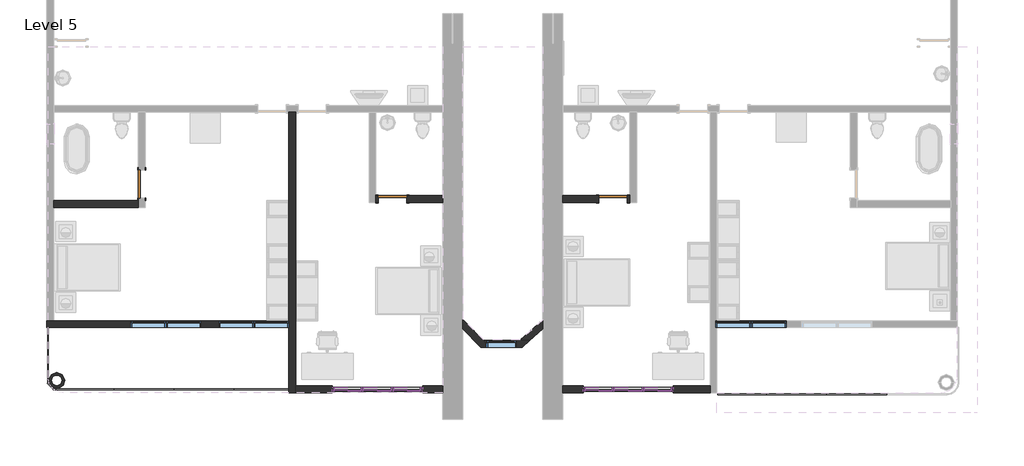
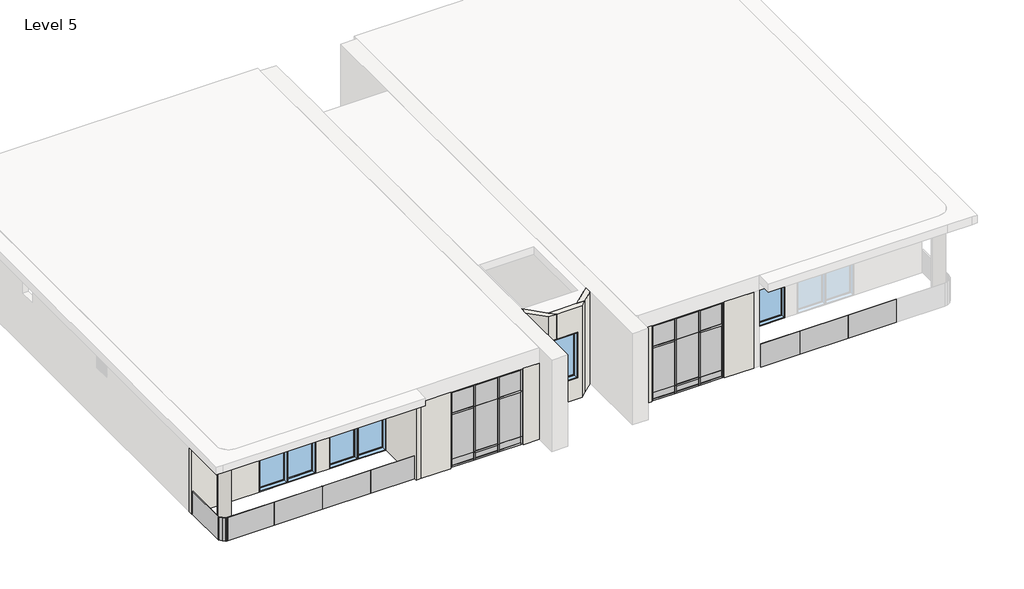
# One storey, part 1 of 3: 42 members, 30 plates, 14 walls, 7 windows, 3 doors.
"""IFC4 building model written with IfcOpenShell, lengths in millimetres."""

from ifc_helpers import new_model, si_unit, point, frame, frame_2d, origin, place, context, project, spatial, polyline, circle_curve, trimmed, segment, composite_curve, outline, extrude, faceted_brep, transform, mapped, element, save
from components import door_2703ae13, door_10fd3a06, member_c17f1be2, member_ad567e07, member_d2e7e466, member_7db1855a, member_75d1e245, member_d60e8053, member_3c3dc66a, member_2fae0574, member_410c6227, member_73c23c35, system_panel_glazed_38d54ecf, system_panel_glazed_fbb6c980, system_panel_glazed_4137532c, system_panel_glazed_6230de04, system_panel_glazed_a79f7f85, system_panel_glazed_9a5ea490, system_panel_glazed_95be5de7, system_panel_glazed_1e00a1c5, system_panel_glazed_ffe51582, system_panel_glazed_8f95e3f6, system_panel_glazed_836907cd, system_panel_glazed_688a65a2, system_panel_glazed_c1a1c740, system_panel_glazed_22bcd51f, window_9a779fa2, window_1a213a25

model = new_model("IFC4")

# Units and contexts
model_context = context("Model", 3, world=origin())
ifc_project = project(units=[si_unit("LENGTHUNIT", "METRE", prefix="MILLI")], contexts=[model_context])

# Site, building, storey
site = spatial("IfcSite", under=ifc_project)
building = spatial("IfcBuilding", under=site)
storey = spatial("IfcBuildingStorey", under=building, Name="Level 5", Elevation=14630.4)

# Doors
placement = place(None, origin())
door_shape = door_2703ae13(model_context)
element("IfcDoor", 1, ObjectType="Door-Single-Panel.0001 : 34\" x 80\"", at=placement, inside=storey, context=model_context, shape_type="MappedRepresentation", body=[
    mapped(door_shape, transform((-15765.9987704, -441.9241442, 14630.4), x_axis=(0.0, -1.0, 0.0), y_axis=(1.0, 0.0, 0.0), z_axis=(0.0, 0.0, 1.0))),
])
element("IfcDoor", 2, ObjectType="Door-Single-Panel.0001 : 34\" x 80\"", at=placement, inside=storey, context=model_context, shape_type="MappedRepresentation", body=[
    mapped(door_shape, transform((-8145.9987704, -899.1241442, 14630.4), x_axis=(-1.0, 0.0, 0.0), y_axis=(0.0, -1.0, 0.0), z_axis=(0.0, 0.0, 1.0))),
])
door_2_shape = door_10fd3a06(model_context)
element("IfcDoor", 3, ObjectType="Door-Single-Panel.0001 : 34\" x 80\"", at=placement, inside=storey, context=model_context, shape_type="MappedRepresentation", body=[
    mapped(door_2_shape, transform((-1440.3987704, -899.1241442, 14630.4), x_axis=(1.0, 0.0, 0.0), y_axis=(0.0, 1.0, 0.0), z_axis=(0.0, 0.0, 1.0))),
])

# Members
member_shape = member_c17f1be2(model_context)
element("IfcMember", 4, ObjectType="Rectangular Mullion : 2.5\" x 5\" rectangular", at=placement, inside=storey, context=model_context, shape_type="MappedRepresentation", body=[
    mapped(member_shape, transform((-9911.2987704, -6690.3241442, 17678.4), x_axis=(0.0, 0.0, 1.0), y_axis=(0.0, 1.0, 0.0), z_axis=(-1.0, 0.0, 0.0))),
])
element("IfcMember", 5, ObjectType="Rectangular Mullion : 2.5\" x 5\" rectangular", at=placement, inside=storey, context=model_context, shape_type="MappedRepresentation", body=[
    mapped(member_shape, transform((-8114.2487704, -6690.3241442, 17678.4), x_axis=(0.0, 0.0, 1.0), y_axis=(0.0, 1.0, 0.0), z_axis=(-1.0, 0.0, 0.0))),
])
element("IfcMember", 6, ObjectType="Rectangular Mullion : 2.5\" x 5\" rectangular", at=placement, inside=storey, context=model_context, shape_type="MappedRepresentation", body=[
    mapped(member_shape, transform((-2291.2987704, -6690.3241442, 17678.4), x_axis=(0.0, 0.0, 1.0), y_axis=(0.0, 1.0, 0.0), z_axis=(-1.0, 0.0, 0.0))),
])
element("IfcMember", 7, ObjectType="Rectangular Mullion : 2.5\" x 5\" rectangular", at=placement, inside=storey, context=model_context, shape_type="MappedRepresentation", body=[
    mapped(member_shape, transform((-494.2487704, -6690.3241442, 17678.4), x_axis=(0.0, 0.0, 1.0), y_axis=(0.0, 1.0, 0.0), z_axis=(-1.0, 0.0, 0.0))),
])
element("IfcMember", 8, ObjectType="Rectangular Mullion : 2.5\" x 5\" rectangular", at=placement, inside=storey, context=model_context, shape_type="MappedRepresentation", body=[
    mapped(member_shape, transform((-7295.0987704, -6690.3241442, 14630.4), x_axis=(0.0, 0.0, -1.0), y_axis=(0.0, 1.0, 0.0), z_axis=(1.0, 0.0, 0.0))),
])
element("IfcMember", 9, ObjectType="Rectangular Mullion : 2.5\" x 5\" rectangular", at=placement, inside=storey, context=model_context, shape_type="MappedRepresentation", body=[
    mapped(member_shape, transform((-9092.1487704, -6690.3241442, 14630.4), x_axis=(0.0, 0.0, -1.0), y_axis=(0.0, 1.0, 0.0), z_axis=(1.0, 0.0, 0.0))),
])
element("IfcMember", 10, ObjectType="Rectangular Mullion : 2.5\" x 5\" rectangular", at=placement, inside=storey, context=model_context, shape_type="MappedRepresentation", body=[
    mapped(member_shape, transform((324.9012296, -6690.3241442, 14630.4), x_axis=(0.0, 0.0, -1.0), y_axis=(0.0, 1.0, 0.0), z_axis=(1.0, 0.0, 0.0))),
])
element("IfcMember", 11, ObjectType="Rectangular Mullion : 2.5\" x 5\" rectangular", at=placement, inside=storey, context=model_context, shape_type="MappedRepresentation", body=[
    mapped(member_shape, transform((-1472.1487704, -6690.3241442, 14630.4), x_axis=(0.0, 0.0, -1.0), y_axis=(0.0, 1.0, 0.0), z_axis=(1.0, 0.0, 0.0))),
])
member_2_shape = member_ad567e07(model_context)
element("IfcMember", 12, ObjectType="Rectangular Mullion : 2.5\" x 5\" rectangular", at=placement, inside=storey, context=model_context, shape_type="MappedRepresentation", body=[
    mapped(member_2_shape, transform((-8114.2487704, -6690.3241442, 16764.0), x_axis=(0.0, 0.0, 1.0), y_axis=(0.0, 1.0, 0.0), z_axis=(-1.0, 0.0, 0.0))),
])
element("IfcMember", 13, ObjectType="Rectangular Mullion : 2.5\" x 5\" rectangular", at=placement, inside=storey, context=model_context, shape_type="MappedRepresentation", body=[
    mapped(member_2_shape, transform((-9911.2987704, -6690.3241442, 16764.0), x_axis=(0.0, 0.0, 1.0), y_axis=(0.0, 1.0, 0.0), z_axis=(-1.0, 0.0, 0.0))),
])
element("IfcMember", 14, ObjectType="Rectangular Mullion : 2.5\" x 5\" rectangular", at=placement, inside=storey, context=model_context, shape_type="MappedRepresentation", body=[
    mapped(member_2_shape, transform((-494.2487704, -6690.3241442, 16764.0), x_axis=(0.0, 0.0, 1.0), y_axis=(0.0, 1.0, 0.0), z_axis=(-1.0, 0.0, 0.0))),
])
element("IfcMember", 15, ObjectType="Rectangular Mullion : 2.5\" x 5\" rectangular", at=placement, inside=storey, context=model_context, shape_type="MappedRepresentation", body=[
    mapped(member_2_shape, transform((-2291.2987704, -6690.3241442, 16764.0), x_axis=(0.0, 0.0, 1.0), y_axis=(0.0, 1.0, 0.0), z_axis=(-1.0, 0.0, 0.0))),
])
member_3_shape = member_d2e7e466(model_context)
element("IfcMember", 16, ObjectType="Rectangular Mullion : 2.5\" x 5\" rectangular", at=placement, inside=storey, context=model_context, shape_type="MappedRepresentation", body=[
    mapped(member_3_shape, transform((-8177.7487704, -6690.3241442, 14630.4), x_axis=(0.0, 0.0, -1.0), y_axis=(0.0, 1.0, 0.0), z_axis=(1.0, 0.0, 0.0))),
])
element("IfcMember", 17, ObjectType="Rectangular Mullion : 2.5\" x 5\" rectangular", at=placement, inside=storey, context=model_context, shape_type="MappedRepresentation", body=[
    mapped(member_3_shape, transform((-557.7487704, -6690.3241442, 14630.4), x_axis=(0.0, 0.0, -1.0), y_axis=(0.0, 1.0, 0.0), z_axis=(1.0, 0.0, 0.0))),
])
member_4_shape = member_7db1855a(model_context)
element("IfcMember", 18, ObjectType="Rectangular Mullion : 2.5\" x 5\" rectangular", at=placement, inside=storey, context=model_context, shape_type="MappedRepresentation", body=[
    mapped(member_4_shape, transform((-9028.6487704, -6690.3241442, 14935.2), x_axis=(0.0, 0.0, 1.0), y_axis=(0.0, 1.0, 0.0), z_axis=(-1.0, 0.0, 0.0))),
])
element("IfcMember", 19, ObjectType="Rectangular Mullion : 2.5\" x 5\" rectangular", at=placement, inside=storey, context=model_context, shape_type="MappedRepresentation", body=[
    mapped(member_4_shape, transform((-1408.6487704, -6690.3241442, 14935.2), x_axis=(0.0, 0.0, 1.0), y_axis=(0.0, 1.0, 0.0), z_axis=(-1.0, 0.0, 0.0))),
])
element("IfcMember", 20, ObjectType="Rectangular Mullion : 2.5\" x 5\" rectangular", at=placement, inside=storey, context=model_context, shape_type="MappedRepresentation", body=[
    mapped(member_3_shape, transform((-9028.6487704, -6690.3241442, 17678.4), x_axis=(0.0, 0.0, 1.0), y_axis=(0.0, 1.0, 0.0), z_axis=(-1.0, 0.0, 0.0))),
])
element("IfcMember", 21, ObjectType="Rectangular Mullion : 2.5\" x 5\" rectangular", at=placement, inside=storey, context=model_context, shape_type="MappedRepresentation", body=[
    mapped(member_3_shape, transform((-1408.6487704, -6690.3241442, 17678.4), x_axis=(0.0, 0.0, 1.0), y_axis=(0.0, 1.0, 0.0), z_axis=(-1.0, 0.0, 0.0))),
])
member_5_shape = member_75d1e245(model_context)
element("IfcMember", 22, ObjectType="Rectangular Mullion : 2.5\" x 5\" rectangular", at=placement, inside=storey, context=model_context, shape_type="MappedRepresentation", body=[
    mapped(member_5_shape, transform((-8145.9987704, -6690.3241442, 14630.4), x_axis=(-1.0, 0.0, 0.0), y_axis=(0.0, 1.0, 0.0), z_axis=(0.0, 0.0, -1.0))),
])
element("IfcMember", 23, ObjectType="Rectangular Mullion : 2.5\" x 5\" rectangular", at=placement, inside=storey, context=model_context, shape_type="MappedRepresentation", body=[
    mapped(member_5_shape, transform((-9060.3987704, -6690.3241442, 14630.4), x_axis=(-1.0, 0.0, 0.0), y_axis=(0.0, 1.0, 0.0), z_axis=(0.0, 0.0, -1.0))),
])
element("IfcMember", 24, ObjectType="Rectangular Mullion : 2.5\" x 5\" rectangular", at=placement, inside=storey, context=model_context, shape_type="MappedRepresentation", body=[
    mapped(member_5_shape, transform((-525.9987704, -6690.3241442, 14630.4), x_axis=(-1.0, 0.0, 0.0), y_axis=(0.0, 1.0, 0.0), z_axis=(0.0, 0.0, -1.0))),
])
element("IfcMember", 25, ObjectType="Rectangular Mullion : 2.5\" x 5\" rectangular", at=placement, inside=storey, context=model_context, shape_type="MappedRepresentation", body=[
    mapped(member_5_shape, transform((-1440.3987704, -6690.3241442, 14630.4), x_axis=(-1.0, 0.0, 0.0), y_axis=(0.0, 1.0, 0.0), z_axis=(0.0, 0.0, -1.0))),
])
member_6_shape = member_d60e8053(model_context)
element("IfcMember", 26, ObjectType="Rectangular Mullion : 2.5\" x 5\" rectangular", at=placement, inside=storey, context=model_context, shape_type="MappedRepresentation", body=[
    mapped(member_6_shape, transform((-8145.9987704, -6690.3241442, 14935.2), x_axis=(-1.0, 0.0, 0.0), y_axis=(0.0, 1.0, 0.0), z_axis=(0.0, 0.0, -1.0))),
])
element("IfcMember", 27, ObjectType="Rectangular Mullion : 2.5\" x 5\" rectangular", at=placement, inside=storey, context=model_context, shape_type="MappedRepresentation", body=[
    mapped(member_6_shape, transform((-9060.3987704, -6690.3241442, 14935.2), x_axis=(-1.0, 0.0, 0.0), y_axis=(0.0, 1.0, 0.0), z_axis=(0.0, 0.0, -1.0))),
])
element("IfcMember", 28, ObjectType="Rectangular Mullion : 2.5\" x 5\" rectangular", at=placement, inside=storey, context=model_context, shape_type="MappedRepresentation", body=[
    mapped(member_6_shape, transform((-525.9987704, -6690.3241442, 14935.2), x_axis=(-1.0, 0.0, 0.0), y_axis=(0.0, 1.0, 0.0), z_axis=(0.0, 0.0, -1.0))),
])
element("IfcMember", 29, ObjectType="Rectangular Mullion : 2.5\" x 5\" rectangular", at=placement, inside=storey, context=model_context, shape_type="MappedRepresentation", body=[
    mapped(member_6_shape, transform((-1440.3987704, -6690.3241442, 14935.2), x_axis=(-1.0, 0.0, 0.0), y_axis=(0.0, 1.0, 0.0), z_axis=(0.0, 0.0, -1.0))),
])
member_7_shape = member_3c3dc66a(model_context)
element("IfcMember", 30, ObjectType="Rectangular Mullion : 2.5\" x 5\" rectangular", at=placement, inside=storey, context=model_context, shape_type="MappedRepresentation", body=[
    mapped(member_7_shape, transform((-9974.7987704, -6690.3241442, 14630.4), x_axis=(-1.0, 0.0, 0.0), y_axis=(0.0, 1.0, 0.0), z_axis=(0.0, 0.0, -1.0))),
])
element("IfcMember", 31, ObjectType="Rectangular Mullion : 2.5\" x 5\" rectangular", at=placement, inside=storey, context=model_context, shape_type="MappedRepresentation", body=[
    mapped(member_7_shape, transform((-2354.7987704, -6690.3241442, 14630.4), x_axis=(-1.0, 0.0, 0.0), y_axis=(0.0, 1.0, 0.0), z_axis=(0.0, 0.0, -1.0))),
])
member_8_shape = member_2fae0574(model_context)
element("IfcMember", 32, ObjectType="Rectangular Mullion : 2.5\" x 5\" rectangular", at=placement, inside=storey, context=model_context, shape_type="MappedRepresentation", body=[
    mapped(member_8_shape, transform((-9974.7987704, -6690.3241442, 14935.2), x_axis=(-1.0, 0.0, 0.0), y_axis=(0.0, 1.0, 0.0), z_axis=(0.0, 0.0, -1.0))),
])
element("IfcMember", 33, ObjectType="Rectangular Mullion : 2.5\" x 5\" rectangular", at=placement, inside=storey, context=model_context, shape_type="MappedRepresentation", body=[
    mapped(member_8_shape, transform((-2354.7987704, -6690.3241442, 14935.2), x_axis=(-1.0, 0.0, 0.0), y_axis=(0.0, 1.0, 0.0), z_axis=(0.0, 0.0, -1.0))),
])
element("IfcMember", 34, ObjectType="Rectangular Mullion : 2.5\" x 5\" rectangular", at=placement, inside=storey, context=model_context, shape_type="MappedRepresentation", body=[
    mapped(member_8_shape, transform((-7231.5987704, -6690.3241442, 16764.0), x_axis=(1.0, 0.0, 0.0), y_axis=(0.0, 1.0, 0.0), z_axis=(0.0, 0.0, 1.0))),
])
element("IfcMember", 35, ObjectType="Rectangular Mullion : 2.5\" x 5\" rectangular", at=placement, inside=storey, context=model_context, shape_type="MappedRepresentation", body=[
    mapped(member_8_shape, transform((388.4012296, -6690.3241442, 16764.0), x_axis=(1.0, 0.0, 0.0), y_axis=(0.0, 1.0, 0.0), z_axis=(0.0, 0.0, 1.0))),
])
element("IfcMember", 36, ObjectType="Rectangular Mullion : 2.5\" x 5\" rectangular", at=placement, inside=storey, context=model_context, shape_type="MappedRepresentation", body=[
    mapped(member_7_shape, transform((-7231.5987704, -6690.3241442, 14935.2), x_axis=(1.0, 0.0, 0.0), y_axis=(0.0, 1.0, 0.0), z_axis=(0.0, 0.0, 1.0))),
])
element("IfcMember", 37, ObjectType="Rectangular Mullion : 2.5\" x 5\" rectangular", at=placement, inside=storey, context=model_context, shape_type="MappedRepresentation", body=[
    mapped(member_7_shape, transform((388.4012296, -6690.3241442, 14935.2), x_axis=(1.0, 0.0, 0.0), y_axis=(0.0, 1.0, 0.0), z_axis=(0.0, 0.0, 1.0))),
])
member_9_shape = member_410c6227(model_context)
element("IfcMember", 38, ObjectType="Rectangular Mullion : 2.5\" x 5\" rectangular", at=placement, inside=storey, context=model_context, shape_type="MappedRepresentation", body=[
    mapped(member_9_shape, transform((-8145.9987704, -6690.3241442, 16764.0), x_axis=(-1.0, 0.0, 0.0), y_axis=(0.0, 1.0, 0.0), z_axis=(0.0, 0.0, -1.0))),
])
element("IfcMember", 39, ObjectType="Rectangular Mullion : 2.5\" x 5\" rectangular", at=placement, inside=storey, context=model_context, shape_type="MappedRepresentation", body=[
    mapped(member_9_shape, transform((-9060.3987704, -6690.3241442, 16764.0), x_axis=(-1.0, 0.0, 0.0), y_axis=(0.0, 1.0, 0.0), z_axis=(0.0, 0.0, -1.0))),
])
element("IfcMember", 40, ObjectType="Rectangular Mullion : 2.5\" x 5\" rectangular", at=placement, inside=storey, context=model_context, shape_type="MappedRepresentation", body=[
    mapped(member_9_shape, transform((-525.9987704, -6690.3241442, 16764.0), x_axis=(-1.0, 0.0, 0.0), y_axis=(0.0, 1.0, 0.0), z_axis=(0.0, 0.0, -1.0))),
])
element("IfcMember", 41, ObjectType="Rectangular Mullion : 2.5\" x 5\" rectangular", at=placement, inside=storey, context=model_context, shape_type="MappedRepresentation", body=[
    mapped(member_9_shape, transform((-1440.3987704, -6690.3241442, 16764.0), x_axis=(-1.0, 0.0, 0.0), y_axis=(0.0, 1.0, 0.0), z_axis=(0.0, 0.0, -1.0))),
])
member_10_shape = member_73c23c35(model_context)
element("IfcMember", 42, ObjectType="Rectangular Mullion : 2.5\" x 5\" rectangular", at=placement, inside=storey, context=model_context, shape_type="MappedRepresentation", body=[
    mapped(member_10_shape, transform((-7231.5987704, -6690.3241442, 17678.4), x_axis=(1.0, 0.0, 0.0), y_axis=(0.0, 1.0, 0.0), z_axis=(0.0, 0.0, 1.0))),
])
element("IfcMember", 43, ObjectType="Rectangular Mullion : 2.5\" x 5\" rectangular", at=placement, inside=storey, context=model_context, shape_type="MappedRepresentation", body=[
    mapped(member_10_shape, transform((388.4012296, -6690.3241442, 17678.4), x_axis=(1.0, 0.0, 0.0), y_axis=(0.0, 1.0, 0.0), z_axis=(0.0, 0.0, 1.0))),
])
element("IfcMember", 44, ObjectType="Rectangular Mullion : 2.5\" x 5\" rectangular", at=placement, inside=storey, context=model_context, shape_type="MappedRepresentation", body=[
    mapped(member_10_shape, transform((-9974.7987704, -6690.3241442, 16764.0), x_axis=(-1.0, 0.0, 0.0), y_axis=(0.0, 1.0, 0.0), z_axis=(0.0, 0.0, -1.0))),
])
element("IfcMember", 45, ObjectType="Rectangular Mullion : 2.5\" x 5\" rectangular", at=placement, inside=storey, context=model_context, shape_type="MappedRepresentation", body=[
    mapped(member_10_shape, transform((-2354.7987704, -6690.3241442, 16764.0), x_axis=(-1.0, 0.0, 0.0), y_axis=(0.0, 1.0, 0.0), z_axis=(0.0, 0.0, -1.0))),
])

# Plates
system_panel_glazed_shape = system_panel_glazed_38d54ecf(model_context)
element("IfcPlate", 46, ObjectType="System Panel : Glazed", at=placement, inside=storey, context=model_context, shape_type="MappedRepresentation", body=[
    mapped(system_panel_glazed_shape, transform((-8603.1987704, -6690.3241442, 14966.95), x_axis=(-1.0, 0.0, 0.0), y_axis=(0.0, -1.0, 0.0), z_axis=(0.0, 0.0, 1.0))),
])
element("IfcPlate", 47, ObjectType="System Panel : Glazed", at=placement, inside=storey, context=model_context, shape_type="MappedRepresentation", body=[
    mapped(system_panel_glazed_shape, transform((-983.1987704, -6690.3241442, 14966.95), x_axis=(-1.0, 0.0, 0.0), y_axis=(0.0, -1.0, 0.0), z_axis=(0.0, 0.0, 1.0))),
])
system_panel_glazed_2_shape = system_panel_glazed_fbb6c980(model_context)
element("IfcPlate", 48, ObjectType="System Panel : Glazed", at=placement, inside=storey, context=model_context, shape_type="MappedRepresentation", body=[
    mapped(system_panel_glazed_2_shape, transform((-8603.1987704, -6690.3241442, 14693.9), x_axis=(-1.0, 0.0, 0.0), y_axis=(0.0, -1.0, 0.0), z_axis=(0.0, 0.0, 1.0))),
])
element("IfcPlate", 49, ObjectType="System Panel : Glazed", at=placement, inside=storey, context=model_context, shape_type="MappedRepresentation", body=[
    mapped(system_panel_glazed_2_shape, transform((-983.1987704, -6690.3241442, 14693.9), x_axis=(-1.0, 0.0, 0.0), y_axis=(0.0, -1.0, 0.0), z_axis=(0.0, 0.0, 1.0))),
])
system_panel_glazed_3_shape = system_panel_glazed_4137532c(model_context)
element("IfcPlate", 50, ObjectType="System Panel : Glazed", at=placement, inside=storey, context=model_context, shape_type="MappedRepresentation", body=[
    mapped(system_panel_glazed_3_shape, transform((-7704.6737704, -6690.3241442, 14693.9), x_axis=(-1.0, 0.0, 0.0), y_axis=(0.0, -1.0, 0.0), z_axis=(0.0, 0.0, 1.0))),
])
element("IfcPlate", 51, ObjectType="System Panel : Glazed", at=placement, inside=storey, context=model_context, shape_type="MappedRepresentation", body=[
    mapped(system_panel_glazed_3_shape, transform((-9501.7237704, -6690.3241442, 14693.9), x_axis=(-1.0, 0.0, 0.0), y_axis=(0.0, -1.0, 0.0), z_axis=(0.0, 0.0, 1.0))),
])
element("IfcPlate", 52, ObjectType="System Panel : Glazed", at=placement, inside=storey, context=model_context, shape_type="MappedRepresentation", body=[
    mapped(system_panel_glazed_3_shape, transform((-84.6737704, -6690.3241442, 14693.9), x_axis=(-1.0, 0.0, 0.0), y_axis=(0.0, -1.0, 0.0), z_axis=(0.0, 0.0, 1.0))),
])
element("IfcPlate", 53, ObjectType="System Panel : Glazed", at=placement, inside=storey, context=model_context, shape_type="MappedRepresentation", body=[
    mapped(system_panel_glazed_3_shape, transform((-1881.7237704, -6690.3241442, 14693.9), x_axis=(-1.0, 0.0, 0.0), y_axis=(0.0, -1.0, 0.0), z_axis=(0.0, 0.0, 1.0))),
])
system_panel_glazed_4_shape = system_panel_glazed_6230de04(model_context)
element("IfcPlate", 54, ObjectType="System Panel : Glazed", at=placement, inside=storey, context=model_context, shape_type="MappedRepresentation", body=[
    mapped(system_panel_glazed_4_shape, transform((-7704.6737704, -6690.3241442, 14935.2), x_axis=(-1.0, 0.0, 0.0), y_axis=(0.0, -1.0, 0.0), z_axis=(0.0, 0.0, 1.0))),
])
element("IfcPlate", 55, ObjectType="System Panel : Glazed", at=placement, inside=storey, context=model_context, shape_type="MappedRepresentation", body=[
    mapped(system_panel_glazed_4_shape, transform((-9501.7237704, -6690.3241442, 14935.2), x_axis=(-1.0, 0.0, 0.0), y_axis=(0.0, -1.0, 0.0), z_axis=(0.0, 0.0, 1.0))),
])
element("IfcPlate", 56, ObjectType="System Panel : Glazed", at=placement, inside=storey, context=model_context, shape_type="MappedRepresentation", body=[
    mapped(system_panel_glazed_4_shape, transform((-84.6737704, -6690.3241442, 14935.2), x_axis=(-1.0, 0.0, 0.0), y_axis=(0.0, -1.0, 0.0), z_axis=(0.0, 0.0, 1.0))),
])
element("IfcPlate", 57, ObjectType="System Panel : Glazed", at=placement, inside=storey, context=model_context, shape_type="MappedRepresentation", body=[
    mapped(system_panel_glazed_4_shape, transform((-1881.7237704, -6690.3241442, 14935.2), x_axis=(-1.0, 0.0, 0.0), y_axis=(0.0, -1.0, 0.0), z_axis=(0.0, 0.0, 1.0))),
])
system_panel_glazed_5_shape = system_panel_glazed_a79f7f85(model_context)
element("IfcPlate", 58, ObjectType="System Panel : Glazed", at=placement, inside=storey, context=model_context, shape_type="MappedRepresentation", body=[
    mapped(system_panel_glazed_5_shape, transform((-7704.6737704, -6690.3241442, 16795.75), x_axis=(-1.0, 0.0, 0.0), y_axis=(0.0, -1.0, 0.0), z_axis=(0.0, 0.0, 1.0))),
])
element("IfcPlate", 59, ObjectType="System Panel : Glazed", at=placement, inside=storey, context=model_context, shape_type="MappedRepresentation", body=[
    mapped(system_panel_glazed_5_shape, transform((-9501.7237704, -6690.3241442, 16795.75), x_axis=(-1.0, 0.0, 0.0), y_axis=(0.0, -1.0, 0.0), z_axis=(0.0, 0.0, 1.0))),
])
element("IfcPlate", 60, ObjectType="System Panel : Glazed", at=placement, inside=storey, context=model_context, shape_type="MappedRepresentation", body=[
    mapped(system_panel_glazed_5_shape, transform((-84.6737704, -6690.3241442, 16795.75), x_axis=(-1.0, 0.0, 0.0), y_axis=(0.0, -1.0, 0.0), z_axis=(0.0, 0.0, 1.0))),
])
element("IfcPlate", 61, ObjectType="System Panel : Glazed", at=placement, inside=storey, context=model_context, shape_type="MappedRepresentation", body=[
    mapped(system_panel_glazed_5_shape, transform((-1881.7237704, -6690.3241442, 16795.75), x_axis=(-1.0, 0.0, 0.0), y_axis=(0.0, -1.0, 0.0), z_axis=(0.0, 0.0, 1.0))),
])
system_panel_glazed_6_shape = system_panel_glazed_9a5ea490(model_context)
element("IfcPlate", 62, ObjectType="System Panel : Glazed", at=placement, inside=storey, context=model_context, shape_type="MappedRepresentation", body=[
    mapped(system_panel_glazed_6_shape, transform((-8603.1987704, -6690.3241442, 16764.0), x_axis=(-1.0, 0.0, 0.0), y_axis=(0.0, -1.0, 0.0), z_axis=(0.0, 0.0, 1.0))),
])
element("IfcPlate", 63, ObjectType="System Panel : Glazed", at=placement, inside=storey, context=model_context, shape_type="MappedRepresentation", body=[
    mapped(system_panel_glazed_6_shape, transform((-983.1987704, -6690.3241442, 16764.0), x_axis=(-1.0, 0.0, 0.0), y_axis=(0.0, -1.0, 0.0), z_axis=(0.0, 0.0, 1.0))),
])
system_panel_glazed_7_shape = system_panel_glazed_95be5de7(model_context)
element("IfcPlate", 64, ObjectType="System Panel : Glazed", at=placement, inside=storey, context=model_context, shape_type="MappedRepresentation", body=[
    mapped(system_panel_glazed_7_shape, transform((-15707.2305745, -6723.6923401, 14630.4), x_axis=(1.0, 0.0, 0.0), y_axis=(0.0, 1.0, 0.0), z_axis=(0.0, 0.0, 1.0))),
])
element("IfcPlate", 65, ObjectType="System Panel : Glazed", at=placement, inside=storey, context=model_context, shape_type="MappedRepresentation", body=[
    mapped(system_panel_glazed_7_shape, transform((-13878.4305745, -6723.6923401, 14630.4), x_axis=(1.0, 0.0, 0.0), y_axis=(0.0, 1.0, 0.0), z_axis=(0.0, 0.0, 1.0))),
])
element("IfcPlate", 66, ObjectType="System Panel : Glazed", at=placement, inside=storey, context=model_context, shape_type="MappedRepresentation", body=[
    mapped(system_panel_glazed_7_shape, transform((5957.9120092, -6810.4133646, 14630.4), x_axis=(-1.0, 0.0, 0.0), y_axis=(0.0, -1.0, 0.0), z_axis=(0.0, 0.0, 1.0))),
])
element("IfcPlate", 67, ObjectType="System Panel : Glazed", at=placement, inside=storey, context=model_context, shape_type="MappedRepresentation", body=[
    mapped(system_panel_glazed_7_shape, transform((4129.1120092, -6810.4133646, 14630.4), x_axis=(-1.0, 0.0, 0.0), y_axis=(0.0, -1.0, 0.0), z_axis=(0.0, 0.0, 1.0))),
])
system_panel_glazed_8_shape = system_panel_glazed_1e00a1c5(model_context)
element("IfcPlate", 68, ObjectType="System Panel : Glazed", at=placement, inside=storey, context=model_context, shape_type="MappedRepresentation", body=[
    mapped(system_panel_glazed_8_shape, transform((2478.1120092, -6810.4133646, 14630.4), x_axis=(-1.0, 0.0, 0.0), y_axis=(0.0, -1.0, 0.0), z_axis=(0.0, 0.0, 1.0))),
])
system_panel_glazed_9_shape = system_panel_glazed_ffe51582(model_context)
element("IfcPlate", 69, ObjectType="System Panel : Glazed", at=placement, inside=storey, context=model_context, shape_type="MappedRepresentation", body=[
    mapped(system_panel_glazed_9_shape, transform((-18451.9713429, -6722.1515718, 14630.4), x_axis=(0.7071067811865462, -0.7071067811865488, 0.0), y_axis=(0.7071067811865488, 0.7071067811865462, 0.0), z_axis=(0.0, 0.0, 1.0))),
])
system_panel_glazed_10_shape = system_panel_glazed_8f95e3f6(model_context)
element("IfcPlate", 70, ObjectType="System Panel : Glazed", at=placement, inside=storey, context=model_context, shape_type="MappedRepresentation", body=[
    mapped(system_panel_glazed_10_shape, transform((-18648.8987704, -5667.9741442, 14630.4), x_axis=(0.0, -1.0, 0.0), y_axis=(1.0, 0.0, 0.0), z_axis=(0.0, 0.0, 1.0))),
])
system_panel_glazed_11_shape = system_panel_glazed_836907cd(model_context)
element("IfcPlate", 71, ObjectType="System Panel : Glazed", at=placement, inside=storey, context=model_context, shape_type="MappedRepresentation", body=[
    mapped(system_panel_glazed_11_shape, transform((-18418.6805745, -6723.6923401, 14630.4), x_axis=(1.0, 0.0, 0.0), y_axis=(0.0, 1.0, 0.0), z_axis=(0.0, 0.0, 1.0))),
])
system_panel_glazed_12_shape = system_panel_glazed_688a65a2(model_context)
element("IfcPlate", 72, ObjectType="System Panel : Glazed", at=placement, inside=storey, context=model_context, shape_type="MappedRepresentation", body=[
    mapped(system_panel_glazed_12_shape, transform((-12129.8146725, -6723.6923401, 14630.4), x_axis=(1.0, 0.0, 0.0), y_axis=(0.0, 1.0, 0.0), z_axis=(0.0, 0.0, 1.0))),
])
system_panel_glazed_13_shape = system_panel_glazed_c1a1c740(model_context)
element("IfcPlate", 73, ObjectType="System Panel : Glazed", at=placement, inside=storey, context=model_context, shape_type="MappedRepresentation", body=[
    mapped(system_panel_glazed_13_shape, transform((-17504.2805745, -6723.6923401, 14630.4), x_axis=(1.0, 0.0, 0.0), y_axis=(0.0, 1.0, 0.0), z_axis=(0.0, 0.0, 1.0))),
])
system_panel_glazed_14_shape = system_panel_glazed_22bcd51f(model_context)
element("IfcPlate", 74, ObjectType="System Panel : Glazed", at=placement, inside=storey, context=model_context, shape_type="MappedRepresentation", body=[
    mapped(system_panel_glazed_14_shape, transform((-18600.0521056, -6574.070809, 14630.4), x_axis=(0.7071067811865462, -0.7071067811865488, 0.0), y_axis=(0.7071067811865488, 0.7071067811865462, 0.0), z_axis=(0.0, 0.0, 1.0))),
])
element("IfcPlate", 75, ObjectType="System Panel : Glazed", at=placement, inside=storey, context=model_context, shape_type="MappedRepresentation", body=[
    mapped(system_panel_glazed_14_shape, transform((-18502.3587761, -6671.7641386, 14630.4), x_axis=(0.7071067811865462, -0.7071067811865488, 0.0), y_axis=(0.7071067811865488, 0.7071067811865462, 0.0), z_axis=(0.0, 0.0, 1.0))),
])

# Walls
element("IfcWall", 76, ObjectType="Generic - 3\" green 2", at=placement, inside=storey, context=model_context, shape_type="SweptSolid", body=[
    extrude(outline(composite_curve([segment(polyline([(-18518.7237704, -6418.8616442), (-18594.9237704, -6418.8616442)]), True, "CONTINUOUS"), segment(trimmed(circle_curve(frame_2d((-18353.6237704, -6418.8616442)), 241.3), [point((-18594.9237704, -6418.8616442))], [point((-18112.3237704, -6418.8616442))], False, "CARTESIAN"), True, "CONTINUOUS"), segment(polyline([(-18112.3237704, -6418.8616442), (-18188.5237704, -6418.8616442)]), True, "CONTINUOUS"), segment(trimmed(circle_curve(frame_2d((-18353.6237704, -6418.8616442)), 165.1), [point((-18188.5237704, -6418.8616442))], [point((-18518.7237704, -6418.8616442))], True, "CARTESIAN"), True, "CONTINUOUS")], self_intersect=False)), frame((0.0, 0.0, 14630.4), z_axis=(0.0, 0.0, 1.0), x_axis=(1.0, 0.0, 0.0)), (0.0, 0.0, 1.0), 3048.0),
])
element("IfcWall", 77, ObjectType="Generic - 3\" green 2", at=placement, inside=storey, context=model_context, shape_type="SweptSolid", body=[
    extrude(outline(composite_curve([segment(polyline([(-18188.5237704, -6418.8616442), (-18112.3237704, -6418.8616442)]), True, "CONTINUOUS"), segment(trimmed(circle_curve(frame_2d((-18353.6237704, -6418.8616442)), 241.3), [point((-18112.3237704, -6418.8616442))], [point((-18594.9237704, -6418.8616442))], False, "CARTESIAN"), True, "CONTINUOUS"), segment(polyline([(-18594.9237704, -6418.8616442), (-18518.7237704, -6418.8616442)]), True, "CONTINUOUS"), segment(trimmed(circle_curve(frame_2d((-18353.6237704, -6418.8616442)), 165.1), [point((-18518.7237704, -6418.8616442))], [point((-18188.5237704, -6418.8616442))], True, "CARTESIAN"), True, "CONTINUOUS")], self_intersect=False)), frame((0.0, 0.0, 14630.4), z_axis=(0.0, 0.0, 1.0), x_axis=(1.0, 0.0, 0.0)), (0.0, 0.0, 1.0), 3048.0),
])
element("IfcWall", 78, ObjectType="Generic - 8\" cream", at=placement, inside=storey, context=model_context, shape_type="Brep", body=[
    faceted_brep([(-11295.5987704, 1742.4758558, 14630.4), (-11295.5987704, -6791.9241442, 14630.4), (-11295.5987704, -6791.9241442, 17678.4), (-11295.5987704, -4810.7241442, 17678.4), (-11295.5987704, -4607.5241442, 17678.4), (-11295.5987704, 1742.4758558, 17678.4), (-11092.3987704, 1742.4758558, 14630.4), (-11092.3987704, 1742.4758558, 17678.4), (-11092.3987704, -6588.7241442, 17678.4), (-11092.3987704, -6791.9241442, 17678.4), (-11092.3987704, -6791.9241442, 14630.4), (-11092.3987704, -6588.7241442, 14630.4)], [[[0, 1, 2, 3, 4, 5]], [[6, 7, 8, 9, 10, 11]], [[1, 0, 6, 11, 10]], [[5, 4, 3, 2, 9, 8, 7]], [[0, 5, 7, 6]], [[2, 1, 10, 9]]]),
])
element("IfcWall", 79, ObjectType="Generic - 8\" cream", at=placement, inside=storey, context=model_context, shape_type="SweptSolid", body=[
    extrude(outline(polyline([(-18445.6987704, -949.9241442), (-15867.5987704, -949.9241442), (-15867.5987704, -1153.1241442), (-18445.6987704, -1153.1241442), (-18445.6987704, -949.9241442)])), frame((0.0, 0.0, 14630.4), z_axis=(0.0, 0.0, 1.0), x_axis=(1.0, 0.0, 0.0)), (0.0, 0.0, 1.0), 3048.0),
])
element("IfcWall", 80, ObjectType="Generic - 8\" cream", at=placement, inside=storey, context=model_context, shape_type="SweptSolid", body=[
    extrude(outline(polyline([(17678.4, -6621.9987704), (17678.4, -8653.9987704), (14630.4, -8653.9987704), (14630.4, -8577.7987704), (16662.4, -8577.7987704), (16662.4, -7714.1987704), (14630.4, -7714.1987704), (14630.4, -6621.9987704), (17678.4, -6621.9987704)])), frame((0.0, -1000.7241442, 0.0), z_axis=(0.0, 1.0, 0.0), x_axis=(0.0, 0.0, 1.0)), (0.0, 0.0, 1.0), 203.2),
])
element("IfcWall", 81, ObjectType="Generic - 8\" cream", at=placement, inside=storey, context=model_context, shape_type="Brep", body=[
    faceted_brep([(-18648.8987704, -4607.5241442, 17678.4), (-18445.6987704, -4607.5241442, 17678.4), (-11295.5987704, -4607.5241442, 17678.4), (-11295.5987704, -4607.5241442, 17373.6), (-13429.1987704, -4607.5241442, 17373.6), (-13429.1987704, -4607.5241442, 14630.4), (-13962.5987704, -4607.5241442, 14630.4), (-13962.5987704, -4607.5241442, 17373.6), (-16096.1987704, -4607.5241442, 17373.6), (-16096.1987704, -4607.5241442, 14630.4), (-18445.6987704, -4607.5241442, 14630.4), (-18648.8987704, -4607.5241442, 14630.4), (-11295.5987704, -4810.7241442, 17678.4), (-18648.8987704, -4810.7241442, 17678.4), (-18648.8987704, -4810.7241442, 14630.4), (-16096.1987704, -4810.7241442, 14630.4), (-16096.1987704, -4810.7241442, 17373.6), (-13962.5987704, -4810.7241442, 17373.6), (-13962.5987704, -4810.7241442, 14630.4), (-13429.1987704, -4810.7241442, 14630.4), (-13429.1987704, -4810.7241442, 17373.6), (-11295.5987704, -4810.7241442, 17373.6)], [[[0, 1, 2, 3, 4, 5, 6, 7, 8, 9, 10, 11]], [[12, 13, 14, 15, 16, 17, 18, 19, 20, 21]], [[14, 11, 10, 9, 15]], [[5, 19, 18, 6]], [[2, 1, 0, 13, 12]], [[2, 12, 21, 3]], [[0, 11, 14, 13]], [[3, 21, 20, 4]], [[4, 20, 19, 5]], [[17, 7, 6, 18]], [[7, 17, 16, 8]], [[8, 16, 15, 9]]]),
])
element("IfcWall", 82, ObjectType="Generic - 8\" cream", at=placement, inside=storey, context=model_context, shape_type="SweptSolid", body=[
    extrude(outline(polyline([(17678.4, -932.3987704), (17678.4, -2964.3987704), (14630.4, -2964.3987704), (14630.4, -1872.1987704), (16662.4, -1872.1987704), (16662.4, -1008.5987704), (14630.4, -1008.5987704), (14630.4, -932.3987704), (17678.4, -932.3987704)])), frame((0.0, -1000.7241442, 0.0), z_axis=(0.0, 1.0, 0.0), x_axis=(0.0, 0.0, 1.0)), (0.0, 0.0, 1.0), 203.2),
])
element("IfcWall", 83, ObjectType="Generic - 8\" cream", at=placement, inside=storey, context=model_context, shape_type="SweptSolid", body=[
    extrude(outline(polyline([(388.4012296, -6588.7241442), (1506.0012296, -6588.7241442), (1506.0012296, -6791.9241442), (388.4012296, -6791.9241442), (388.4012296, -6588.7241442)])), frame((0.0, 0.0, 14630.4), z_axis=(0.0, 0.0, 1.0), x_axis=(1.0, 0.0, 0.0)), (0.0, 0.0, 1.0), 3048.0),
])
element("IfcWall", 84, ObjectType="Generic - 8\" cream", at=placement, inside=storey, context=model_context, shape_type="SweptSolid", body=[
    extrude(outline(polyline([(-2354.7987704, -6791.9241442), (-2964.3987704, -6791.9241442), (-2964.3987704, -6588.7241442), (-2354.7987704, -6588.7241442), (-2354.7987704, -6791.9241442)])), frame((0.0, 0.0, 14630.4), z_axis=(0.0, 0.0, 1.0), x_axis=(1.0, 0.0, 0.0)), (0.0, 0.0, 1.0), 3048.0),
])
element("IfcWall", 85, ObjectType="Generic - 8\" cream", at=placement, inside=storey, context=model_context, shape_type="SweptSolid", body=[
    extrude(outline(polyline([(-9974.7987704, -6791.9241442), (-11092.3987704, -6791.9241442), (-11092.3987704, -6588.7241442), (-9974.7987704, -6588.7241442), (-9974.7987704, -6791.9241442)])), frame((0.0, 0.0, 14630.4), z_axis=(0.0, 0.0, 1.0), x_axis=(1.0, 0.0, 0.0)), (0.0, 0.0, 1.0), 3048.0),
])
element("IfcWall", 86, ObjectType="Generic - 8\" cream", at=placement, inside=storey, context=model_context, shape_type="SweptSolid", body=[
    extrude(outline(polyline([(-7231.5987704, -6588.7241442), (-6621.9987704, -6588.7241442), (-6621.9987704, -6791.9241442), (-7231.5987704, -6791.9241442), (-7231.5987704, -6588.7241442)])), frame((0.0, 0.0, 14630.4), z_axis=(0.0, 0.0, 1.0), x_axis=(1.0, 0.0, 0.0)), (0.0, 0.0, 1.0), 3048.0),
])
element("IfcWall", 87, ObjectType="Generic - 8\" green", at=placement, inside=storey, context=model_context, shape_type="Brep", body=[
    faceted_brep([(-6012.3987704, -4852.8082422, 14630.4), (-5458.7044276, -5406.502585, 14630.4), (-5458.7044276, -5406.502585, 18288.0), (-6012.3987704, -4852.8082422, 18288.0), (-5171.3362318, -5406.502585, 14630.4), (-5374.5362318, -5203.302585, 14630.4), (-6012.3987704, -4565.4400463, 14630.4), (-6012.3987704, -4565.4400463, 18288.0), (-5374.5362318, -5203.302585, 18288.0), (-5171.3362318, -5406.502585, 18288.0), (-5171.3362318, -5406.502585, 17297.4), (-5289.4901401, -5288.3486766, 17297.4), (-5289.4901401, -5288.3486766, 15468.6), (-5171.3362318, -5406.502585, 15468.6), (-5289.4901401, -5406.502585, 15468.6), (-5289.4901401, -5406.502585, 17297.4)], [[[0, 1, 2, 3]], [[4, 5, 6, 7, 8, 9, 10, 11, 12, 13]], [[1, 0, 6, 5, 4]], [[3, 2, 9, 8, 7]], [[0, 3, 7, 6]], [[2, 1, 4, 13, 14, 15, 10, 9]], [[12, 14, 13]], [[14, 12, 11, 15]], [[15, 11, 10]]]),
])
element("IfcWall", 88, ObjectType="Generic - 8\" green", at=placement, inside=storey, context=model_context, shape_type="Brep", body=[
    faceted_brep([(-5171.3362318, -5406.502585, 14630.4), (-4203.3343712, -5406.502585, 14630.4), (-4203.3343712, -5406.502585, 18288.0), (-5171.3362318, -5406.502585, 18288.0), (-5171.3362318, -5406.502585, 17297.4), (-4375.0901401, -5406.502585, 17297.4), (-4375.0901401, -5406.502585, 15468.6), (-5171.3362318, -5406.502585, 15468.6), (-3975.4820774, -5203.302585, 14630.4), (-4280.7801413, -5203.302585, 14630.4), (-5374.5362318, -5203.302585, 14630.4), (-5374.5362318, -5203.302585, 18288.0), (-4280.7801413, -5203.302585, 18288.0), (-3975.4820774, -5203.302585, 18288.0), (-4375.0901401, -5203.302585, 15468.6), (-4375.0901401, -5203.302585, 17297.4), (-5289.4901401, -5203.302585, 17297.4), (-5289.4901401, -5203.302585, 15468.6), (-5289.4901401, -5288.3486766, 15468.6), (-5289.4901401, -5288.3486766, 17297.4)], [[[0, 1, 2, 3, 4, 5, 6, 7]], [[8, 9, 10, 11, 12, 13], [14, 15, 16, 17]], [[1, 0, 10, 9, 8]], [[3, 2, 13, 12, 11]], [[3, 11, 10, 0, 7, 18, 19, 4]], [[2, 1, 8, 13]], [[5, 15, 14, 6]], [[6, 14, 17, 18, 7]], [[18, 17, 16, 19]], [[15, 5, 4, 19, 16]]]),
])
element("IfcWall", 89, ObjectType="Generic - 8\" green", at=placement, inside=storey, context=model_context, shape_type="SweptSolid", body=[
    extrude(outline(polyline([(-3573.9987704, -4845.2574382), (-3975.4820774, -5203.302585), (-4280.7801413, -5203.302585), (-3573.9987704, -4572.9908503), (-3573.9987704, -4845.2574382)])), frame((0.0, 0.0, 14630.4), z_axis=(0.0, 0.0, 1.0), x_axis=(1.0, 0.0, 0.0)), (0.0, 0.0, 1.0), 3657.6),
])

# Windows
window_shape = window_9a779fa2(model_context)
element("IfcWindow", 90, ObjectType="Fixed : 36\" x 72\"", at=placement, inside=storey, context=model_context, shape_type="MappedRepresentation", body=[
    mapped(window_shape, transform((-4794.1901401, -5304.902585, 15163.8), x_axis=(1.0, 0.0, 0.0), y_axis=(0.0, 1.0, 0.0), z_axis=(0.0, 0.0, 1.0))),
])
window_2_shape = window_1a213a25(model_context)
element("IfcWindow", 91, ObjectType="Fixed : 36\" x 72\" 2", at=placement, inside=storey, context=model_context, shape_type="MappedRepresentation", body=[
    mapped(window_2_shape, transform((-11790.8987704, -4709.1241442, 14325.6), x_axis=(1.0, 0.0, 0.0), y_axis=(0.0, 1.0, 0.0), z_axis=(0.0, 0.0, 1.0))),
])
element("IfcWindow", 92, ObjectType="Fixed : 36\" x 72\" 2", at=placement, inside=storey, context=model_context, shape_type="MappedRepresentation", body=[
    mapped(window_2_shape, transform((-12857.6987704, -4709.1241442, 14325.6), x_axis=(1.0, 0.0, 0.0), y_axis=(0.0, 1.0, 0.0), z_axis=(0.0, 0.0, 1.0))),
])
element("IfcWindow", 93, ObjectType="Fixed : 36\" x 72\" 2", at=placement, inside=storey, context=model_context, shape_type="MappedRepresentation", body=[
    mapped(window_2_shape, transform((-14457.8987704, -4709.1241442, 14325.6), x_axis=(1.0, 0.0, 0.0), y_axis=(0.0, 1.0, 0.0), z_axis=(0.0, 0.0, 1.0))),
])
element("IfcWindow", 94, ObjectType="Fixed : 36\" x 72\" 2", at=placement, inside=storey, context=model_context, shape_type="MappedRepresentation", body=[
    mapped(window_2_shape, transform((-15524.6987704, -4709.1241442, 14325.6), x_axis=(1.0, 0.0, 0.0), y_axis=(0.0, 1.0, 0.0), z_axis=(0.0, 0.0, 1.0))),
])
element("IfcWindow", 95, ObjectType="Fixed : 36\" x 72\" 2", at=placement, inside=storey, context=model_context, shape_type="MappedRepresentation", body=[
    mapped(window_2_shape, transform((2255.3012296, -4709.1241442, 14325.6), x_axis=(1.0, 0.0, 0.0), y_axis=(0.0, 1.0, 0.0), z_axis=(0.0, 0.0, 1.0))),
])
element("IfcWindow", 96, ObjectType="Fixed : 36\" x 72\" 2", at=placement, inside=storey, context=model_context, shape_type="MappedRepresentation", body=[
    mapped(window_2_shape, transform((3331.6262296, -4709.1241442, 14325.6), x_axis=(1.0, 0.0, 0.0), y_axis=(0.0, 1.0, 0.0), z_axis=(0.0, 0.0, 1.0))),
])

save(model, "model.ifc")

# Revit data of these elements
# Type "Door-Single-Panel.0001 : 34\" x 80\""
#   Type Mark = "9"
#   Construction Type Id = "DOOR"
#   Assembly Code = "C1020300"
#   Analytic Construction = "Wooden"
#   Thickness = 0' - 2"
#   Thermal Resistance (R) = 0.455703 (m²·K)/W
#   Swing Angle [instance default] = 90.00°
#   Heat Transfer Coefficient (U) = 2.19465 W/(m²·K)
#   Height = 6' - 8"
#   Trim Projection Ext = 0' - 1"
#   Trim Projection Int = 0' - 1"
#   Trim Width = 0' - 3"
#   Width = 2' - 10"
#   Panel Material = Wood - Birch - Solid Stained Light Low Gloss
#   Trim Material = Paint - Sienna
#   Visual Light Transmittance = 0
#   Solar Heat Gain Coefficient = 0
#   Function = (empty or 0)
#   Wall Closure = (empty or 0)
# Type "Rectangular Mullion : 2.5\" x 5\" rectangular"
#   built-in parameter 1007304 = 0.416667 (stored number, unit not read)
#   built-in parameter 1007301 = 0.104167 (stored number, unit not read)
#   built-in parameter 1007300 = 0.104167 (stored number, unit not read)
# Type "System Panel : Glazed"
#   Construction Type Id = "GSP4R"
#   Analytic Construction = "1/8 in Pilkington single glazing"
#   Visual Light Transmittance = 0.9
#   Solar Heat Gain Coefficient = 0.86
#   Heat Transfer Coefficient (U) = 6.7069 W/(m²·K)
# Type "Generic - 3\" green 2"
#   Assembly Code = "B2010"
#   Width = 0' - 3"
#   Layers, outside or top first: 0' - 3" "Damp-proofing" (function 1)
# Type "Generic - 8\" cream"
#   Assembly Code = "B2010"
#   Width = 0' - 8"
#   Layers, outside or top first: 0' - 8" "Parking Stripe" (function 1)
# Type "Generic - 8\" green"
#   Assembly Code = "B2010"
#   Width = 0' - 8"
#   Layers, outside or top first: 0' - 8" "Damp-proofing" (function 1)
# Type "Fixed : 36\" x 72\""
#   Type Mark = "9"
#   Construction Type Id = "GSP4R"
#   Assembly Code = "B2020100"
#   Analytic Construction = "1/8 in Pilkington single glazing"
#   Visual Light Transmittance = 0.9
#   Solar Heat Gain Coefficient = 0.78
#   Heat Transfer Coefficient (U) = 3.6886 W/(m²·K)
#   Height = 6' - 0"
#   Default Sill Height = 1' - 0"
#   Width = 3' - 0"
#   Window Inset = 0' - 0 3/4"
#   Glass Pane Material = Glass
#   Sash Material = Iron, Ductile
#   Wall Closure = (empty or 0)
# Type "Fixed : 36\" x 72\" 2"
#   Type Mark = "29"
#   Construction Type Id = "GSP4R"
#   Assembly Code = "B2020100"
#   Analytic Construction = "1/8 in Pilkington single glazing"
#   Visual Light Transmittance = 0.9
#   Solar Heat Gain Coefficient = 0.78
#   Heat Transfer Coefficient (U) = 3.6886 W/(m²·K)
#   Height = 9' - 0"
#   Default Sill Height = 1' - 0"
#   Width = 3' - 6"
#   Window Inset = 0' - 0 3/4"
#   Glass Pane Material = Glass
#   Sash Material = Iron, Ductile
#   Wall Closure = (empty or 0)
# Elements 1, 2, 3 (IfcDoor, "Door-Single-Panel.0001 : 34\" x 80\"")
#   Swing Angle = 90.00°
#   Phase Created = New Construction
#   Materials on its faces: "Paint - Sienna", "Wood - Birch - Solid Stained Light Low Gloss"
# Elements 4, 5, 6, 7, 8, 9, 10, 11, 12, 13, 14, 15, 16, 17, 18, 19, 20, 21, 22, 23, 24, 25, 26, 27, 28, 29, 30, 31, 32, 33, 34, 35, 36, 37, 38, 39, 40, 41, 42, 43, 44, 45 (IfcMember, "Rectangular Mullion : 2.5\" x 5\" rectangular")
#   Phase Created = New Construction
#   Materials on its faces: "Iron, Ductile"
# Elements 46, 47, 48, 49, 50, 51, 52, 53, 54, 55, 56, 57, 58, 59, 60, 61, 62, 63, 64, 65, 66, 67, 68, 69, 70, 71, 72, 73, 74, 75 (IfcPlate, "System Panel : Glazed")
#   Phase Created = New Construction
#   Materials on its faces: "Glass"
# Elements 76, 77 (IfcWall, "Generic - 3\" green 2")
#   Top Offset = 0' - 0"
#   Base Offset = 0' - 0"
#   Unconnected Height = 10' - 0"
#   wall height = 10' - 0"
#   Phase Created = New Construction
#   Materials on its faces: "Damp-proofing"
# Elements 78, 79, 80, 81, 82, 83, 84, 85, 86 (IfcWall, "Generic - 8\" cream")
#   Top Offset = 0' - 0"
#   Base Offset = 0' - 0"
#   Unconnected Height = 10' - 0"
#   wall height = 10' - 0"
#   Phase Created = New Construction
#   Base Constraint = Level 5
#   Materials on its faces: "Parking Stripe"
# Elements 87, 88, 89 (IfcWall, "Generic - 8\" green")
#   Top Offset = 0' - 0"
#   Base Offset = 0' - 0"
#   Unconnected Height = 12' - 0"
#   wall height = 12' - 0"
#   Phase Created = New Construction
#   Base Constraint = Level 5
#   Materials on its faces: "Damp-proofing"
# Element 90 (IfcWindow, "Fixed : 36\" x 72\"")
#   Mark = "131"
#   Phase Created = New Construction
#   Materials on its faces: "Iron, Ductile", "Glass"
# Element 91 (IfcWindow, "Fixed : 36\" x 72\" 2")
#   Mark = "132"
#   Phase Created = New Construction
#   Materials on its faces: "Iron, Ductile", "Glass"
# Element 92 (IfcWindow, "Fixed : 36\" x 72\" 2")
#   Mark = "133"
#   Phase Created = New Construction
#   Materials on its faces: "Iron, Ductile", "Glass"
# Element 93 (IfcWindow, "Fixed : 36\" x 72\" 2")
#   Mark = "134"
#   Phase Created = New Construction
#   Materials on its faces: "Iron, Ductile", "Glass"
# Element 94 (IfcWindow, "Fixed : 36\" x 72\" 2")
#   Mark = "135"
#   Phase Created = New Construction
#   Materials on its faces: "Iron, Ductile", "Glass"
# Element 95 (IfcWindow, "Fixed : 36\" x 72\" 2")
#   Mark = "136"
#   Phase Created = New Construction
#   Materials on its faces: "Iron, Ductile", "Glass"
# Element 96 (IfcWindow, "Fixed : 36\" x 72\" 2")
#   Mark = "137"
#   Phase Created = New Construction
#   Materials on its faces: "Iron, Ductile", "Glass"
# Materials
#   "Wood - Birch - Solid Stained Light Low Gloss": class "Wood", colour RGB 210 159 95, transparency 0, Cost = 0
#   "Paint - Sienna": colour RGB 118 70 51, transparency 0, Cost = 0
#   "Damp-proofing": class "Generic", colour RGB 127 127 127, transparency 0, Description = "Damp-proofing", Cost = 0
#   "Parking Stripe": class "Paint", colour RGB 250 250 91, transparency 0, Cost = 0
#   "Glass": class "Glass", colour RGB 0 128 192, transparency 0.75, Description = "Soda Lime Glass", Cost = 0
#   "Iron, Ductile": class "Metal", colour RGB 0 0 0, transparency 0, Description = "Ductile cast iron", Cost = 0
